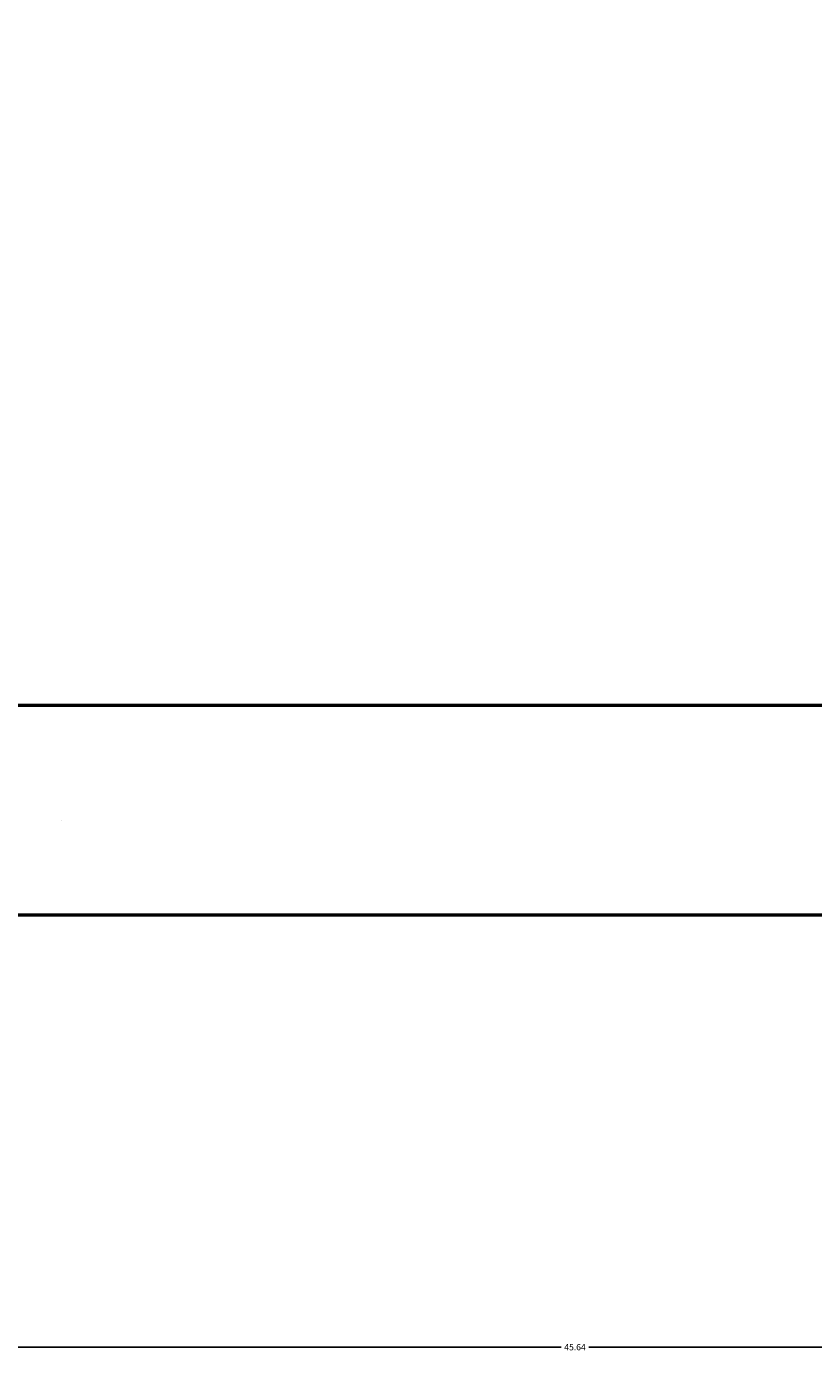
# Model space of a CAD drawing. Units: inches. Extents: x 2812 to 3051, y 1398 to 1659.
# Tile 3 of 65: x 2858 to 2880, y 1398 to 1435. Entities that reach past the tile are written whole.
import ezdxf

# ---------------------------------------------------------------- set-up
doc = ezdxf.new("R2010")
doc.units = ezdxf.units.IN
for name, color, linetype, lineweight in [('A-ANNO-DIMS', 2, 'Continuous', 18), ('S-CONC', 7, 'Continuous', 50), ('S-CONC-PATT', 8, 'Continuous', 18)]:
    doc.layers.add(name, color=color, linetype=linetype, lineweight=lineweight)
doc.styles.get("Standard").update_dxf_attribs({"font": 'arial.ttf'})
doc.dimstyles.get("Standard").update_dxf_attribs({"dimtxt": 0.18, "dimasz": 0.18, "dimexe": 0.18, "dimexo": 0.0625, "dimgap": 0.09, "dimtad": 0, "dimtih": 1, "dimtoh": 1, "dimdec": 4, "dimzin": 0, "dimdsep": 46, "dimtxsty": 'Standard', "dimcen": 0.09, "dimadec": 0, "dimazin": 0, "dimtfac": 1, "dimtdec": 4, "dimtofl": 0, "dimtmove": 0, "dimatfit": 3, "dimfxl": 1, "dimtolj": 1, "dimtzin": 0, "dimarcsym": 0})

# ---------------------------------------------------------------- blocks, each defined once
blk = doc.blocks.new('*D44')
at = {"layer": 'A-ANNO-DIMS', "color": 0, "lineweight": -2, "transparency": 16777216}
for p, q in [((2850.748, 1487.973), (2850.748, 1397.505)), ((2896.385, 1487.973), (2896.385, 1397.505)), ((2850.928, 1397.685), (2873.17, 1397.685)), ((2896.205, 1397.685), (2873.964, 1397.685))]:
    blk.add_line(p, q, dxfattribs=at)
at = {"layer": 'A-ANNO-DIMS', "color": 0, "transparency": 16777216}
for points in [[(2850.928, 1397.715), (2850.928, 1397.655), (2850.748, 1397.685)], [(2896.205, 1397.715), (2896.205, 1397.655), (2896.385, 1397.685)]]:
    blk.add_solid(points, dxfattribs=at)
at = {"layer": 'Defpoints', "color": 0, "transparency": 16777216}
for p in [(2850.748, 1488.035), (2896.385, 1488.035), (2896.385, 1397.685)]:
    blk.add_point(p, dxfattribs=at)
at = {"layer": 'A-ANNO-DIMS', "color": 0, "transparency": 16777216, "insert": (2873.567, 1397.685), "char_height": 0.18, "attachment_point": 5}
blk.add_mtext('\\A1;45.64', dxfattribs=at)
blk = doc.blocks.new('*D56')
at = {"layer": 'A-ANNO-DIMS', "color": 0, "lineweight": -2, "transparency": 16777216}
for p, q in [((2880.322, 1452.035), (2811.806, 1452.035)), ((2811.986, 1451.855), (2811.986, 1434.217)), ((2811.986, 1416.215), (2811.986, 1433.853)), ((2952.322, 1416.035), (2811.806, 1416.035))]:
    blk.add_line(p, q, dxfattribs=at)
at = {"layer": 'A-ANNO-DIMS', "color": 0, "transparency": 16777216}
for points in [[(2811.956, 1451.855), (2812.016, 1451.855), (2811.986, 1452.035)], [(2811.956, 1416.215), (2812.016, 1416.215), (2811.986, 1416.035)]]:
    blk.add_solid(points, dxfattribs=at)
at = {"layer": 'Defpoints', "color": 0, "transparency": 16777216}
for p in [(2811.986, 1452.035), (2880.385, 1452.035), (2952.385, 1416.035)]:
    blk.add_point(p, dxfattribs=at)
at = {"layer": 'A-ANNO-DIMS', "color": 0, "transparency": 16777216, "insert": (2811.986, 1434.035), "char_height": 0.18, "attachment_point": 5}
blk.add_mtext('\\A1;36', dxfattribs=at)
blk = doc.blocks.new('*D75')
at = {"layer": 'A-ANNO-DIMS', "color": 0, "lineweight": -2, "transparency": 16777216}
for p, q in [((2963.812, 1448.474), (2811.806, 1448.474)), ((2811.986, 1448.294), (2811.986, 1432.437)), ((2811.986, 1416.215), (2811.986, 1432.073)), ((2961.322, 1416.035), (2811.806, 1416.035))]:
    blk.add_line(p, q, dxfattribs=at)
at = {"layer": 'A-ANNO-DIMS', "color": 0, "transparency": 16777216}
for points in [[(2811.956, 1448.294), (2812.016, 1448.294), (2811.986, 1448.474)], [(2811.956, 1416.215), (2812.016, 1416.215), (2811.986, 1416.035)]]:
    blk.add_solid(points, dxfattribs=at)
at = {"layer": 'Defpoints', "color": 0, "transparency": 16777216}
for p in [(2811.986, 1448.474), (2963.874, 1448.474), (2961.385, 1416.035)]:
    blk.add_point(p, dxfattribs=at)
at = {"layer": 'A-ANNO-DIMS', "color": 0, "transparency": 16777216, "insert": (2811.986, 1432.255), "char_height": 0.18, "attachment_point": 5}
blk.add_mtext('\\A1;32.44', dxfattribs=at)

msp = doc.modelspace()

# ---------------------------------------------------------------- hatches: boundary and pattern name
at = {"layer": 'S-CONC-PATT'}
h = msp.add_hatch(dxfattribs=at)
h.set_pattern_fill('AR-SAND', color=256, scale=0.3)
h.paths.add_polyline_path([(3036.3849, 1416.0354), (3027.3849, 1416.0354), (2826.3849, 1416.0354), (2826.3849, 1410.0354), (2835.3849, 1410.0354), (3036.3849, 1410.0354)])
h.paths.add_polyline_path([(2970.3849, 1488.0354), (2969.3849, 1488.0354), (2941.3849, 1488.0354), (2941.3849, 1482.0354), (2970.3849, 1482.0354)])
h.paths.add_polyline_path([(3036.3849, 1488.0354), (3035.3849, 1488.0354), (3006.3849, 1488.0354), (3006.3849, 1482.0354), (3027.3849, 1482.0354), (3036.3849, 1482.0354)])
h.paths.add_polyline_path([(3034.3849, 1490.0354), (3008.3849, 1490.0354), (3008.3849, 1489.0354), (3034.3849, 1489.0354)])
h.paths.add_polyline_path([(3035.3849, 1489.0354), (3034.3849, 1489.0354), (3007.3849, 1489.0354), (3007.3849, 1488.0354), (3035.3849, 1488.0354)])
h.paths.add_polyline_path([(2968.3849, 1490.0354), (2943.3849, 1490.0354), (2943.3849, 1489.0354), (2968.3849, 1489.0354)])
h.paths.add_polyline_path([(2969.3849, 1489.0354), (2968.3849, 1489.0354), (2942.3849, 1489.0354), (2942.3849, 1488.0354), (2969.3849, 1488.0354)])
h.paths.add_polyline_path([(2896.3849, 1488.0354), (2826.3849, 1488.0354), (2826.3849, 1482.0354), (2896.3849, 1482.0354)])
h.paths.add_polyline_path([(2895.3849, 1489.0354), (2894.3849, 1489.0354), (2827.3849, 1489.0354), (2827.3849, 1488.0354), (2895.3849, 1488.0354)])
h.paths.add_polyline_path([(2894.3849, 1490.0354), (2828.3849, 1490.0354), (2828.3849, 1489.0354), (2894.3849, 1489.0354)])
h = msp.add_hatch(dxfattribs=at)
h.set_pattern_fill('AR-CONC', color=256, scale=0.3)
h.paths.add_polyline_path([(3036.3849, 1416.0354), (3027.3849, 1416.0354), (2826.3849, 1416.0354), (2826.3849, 1410.0354), (2835.3849, 1410.0354), (3036.3849, 1410.0354)])

# ---------------------------------------------------------------- linework, layer by layer
at = {"layer": 'S-CONC'}
for p, q in [((2826.3849, 1416.0354), (3027.3849, 1416.0354)), ((2835.3849, 1410.0354), (3036.3849, 1410.0354))]:
    msp.add_line(p, q, dxfattribs=at)

# ---------------------------------------------------------------- dimensions: what is measured, and where the dimension line sits
at = {"layer": 'A-ANNO-DIMS'}
dim = msp.add_linear_dim(base=(2896.3849, 1397.6854), p1=(2850.7485, 1488.0354), p2=(2896.3849, 1488.0354), dimstyle='Standard', override={"dimdec": 2, "dimlfac": 1, "dimrnd": 0, "dimzin": 0, "dimdsep": 46, "dimlunit": 2}, dxfattribs=at)
dim.commit()
dim.dimension.update_dxf_attribs({"geometry": '*D44', "text_midpoint": (2873.5667, 1397.6854)})
for base, p1, p2, override, picture, middle in [((2811.9855, 1452.0354), (2952.3849, 1416.0354), (2880.3849, 1452.0354), {"dimdec": 0, "dimlfac": 1, "dimrnd": 0, "dimzin": 0, "dimdsep": 46, "dimlunit": 2}, '*D56', (2811.9855, 1434.0354)), ((2811.9855, 1448.4738), (2961.3849, 1416.0354), (2963.8741, 1448.4738), {"dimdec": 2, "dimlfac": 1, "dimrnd": 0, "dimzin": 0, "dimdsep": 46, "dimlunit": 2}, '*D75', (2811.9855, 1432.2546))]:
    dim = msp.add_linear_dim(base=base, p1=p1, p2=p2, angle=90, dimstyle='Standard', override=override, dxfattribs=at)
    dim.commit()
    dim.dimension.update_dxf_attribs({"geometry": picture, "text_midpoint": middle})

doc.saveas('drawing.dxf')
